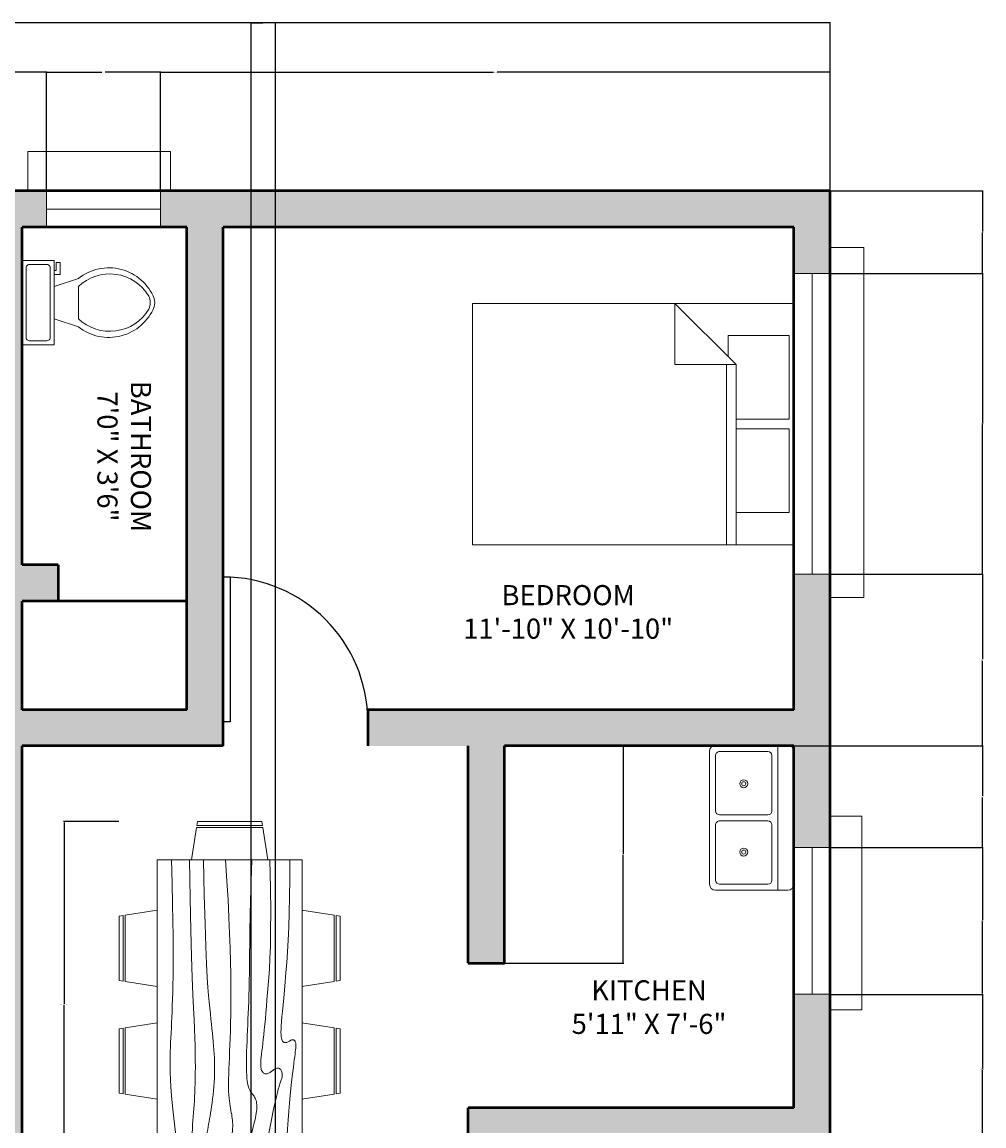
# Model space of a CAD drawing. Units: inches. Extents: x 2710 to 3197, y 524 to 1147.
# Tile 6 of 6: x 2957 to 3197, y 873 to 1147. Entities that reach past the tile are written whole.
import ezdxf

# ---------------------------------------------------------------- set-up
doc = ezdxf.new("R2010")
doc.units = ezdxf.units.IN
for name, color, linetype, lineweight in [('A-ANNO-DIMS', 2, 'Continuous', 18), ('A-AREA-IDEN', 7, 'Continuous', 25), ('A-DOOR', 3, 'Continuous', 25), ('A-FLOR-FIXT', 9, 'Continuous', 20), ('A-FURN', 8, 'Continuous', 18), ('A-GLAZ', 4, 'Continuous', 18), ('A-WALL', 7, 'Continuous', 50), ('A-WALL-PATT', 74, 'Continuous', 13)]:
    doc.layers.add(name, color=color, linetype=linetype, lineweight=lineweight)
doc.styles.get("Standard").update_dxf_attribs({"font": 'arial.ttf'})
doc.dimstyles.get("Standard").update_dxf_attribs({"dimtxt": 0.18, "dimasz": 0.18, "dimexe": 0.18, "dimexo": 0.0625, "dimgap": 0.09, "dimtad": 0, "dimtih": 1, "dimtoh": 1, "dimdec": 4, "dimzin": 0, "dimdsep": 46, "dimtxsty": 'Standard', "dimcen": 0.09, "dimadec": 0, "dimazin": 0, "dimtfac": 1, "dimtdec": 4, "dimtofl": 0, "dimtmove": 0, "dimatfit": 3, "dimfxl": 1, "dimtolj": 1, "dimtzin": 0, "dimarcsym": 0})

# ---------------------------------------------------------------- blocks, each defined once
blk = doc.blocks.new('*U4')
for p, q in [((0, 0), (0, -6)), ((36, 0), (36, -6))]:
    blk.add_line(p, q)
blk.add_lwpolyline([(0, 0), (0, 36), (1.75, 36), (1.75, 0)], close=True)
blk.add_arc((0, 0), 36, 0, 90)
blk = doc.blocks.new('Bed - Queen')
for p, q in [((0, -80.00003), (0, 0)), ((0, 0), (59.99999, 0)), ((59.99999, 0), (59.99999, -80.00003)), ((7.99999, -1.2), (28.79998, -1.2)), ((7.99999, -14.4), (7.99999, -1.2)), ((28.79998, -1.2), (28.79998, -14.4)), ((31.19999, -1.2), (51.99999, -1.2)), ((31.19999, -14.4), (31.19999, -1.2)), ((51.99999, -1.2), (51.99999, -16.4)), ((0, -14.4), (44.8, -14.4)), ((59.99999, -29.6), (44.8, -14.4)), ((44.8, -14.4), (44.8, -29.6)), ((51.99999, -16.4), (46.79936, -16.4)), ((44.8, -16.8), (0, -16.8)), ((44.8, -29.6), (59.99999, -29.6)), ((59.99999, -80.00003), (0, -80.00003))]:
    blk.add_line(p, q)
blk = doc.blocks.new('Toilet - top')
for p, q in [((9.5, -6), (9.5, -2)), ((-8, -8.5), (-8, -8)), ((-7, -8), (-7, -9.5)), ((-4, -8), (-6, -14)), ((4, -8), (6, -14)), ((-10, -8.5), (-8, -8.5)), ((-10, -9.5), (-10, -8.5)), ((-7, -9.5), (-10, -9.5)), ((4, -14), (-4, -14))]:
    blk.add_line(p, q)
blk.add_lwpolyline([(10.5, -8), (10.5, 0), (-10.5, 0), (-10.5, -8)], close=True)
for points in [[(-9.5, -2), (-9.5, -6)], [(8.5, -1), (-8.5, -1)], [(-8.5, -7), (8.5, -7)]]:
    blk.add_lwpolyline(points)
for centre, radius, start, end in [((-8.62, -1.88), 0.884, 81.8699, 188.1301), ((8.62, -1.88), 0.884, 351.8699, 98.1301), ((-8.62, -6.12), 0.884, 171.8699, 278.1301), ((8.62, -6.12), 0.884, 261.8699, 8.1301), ((3.52, -21.58), 12.17, 141.4691, 247.9714), ((4.2, -21.82), 11.33, 136.3677, 238.9468), ((-3.52, -21.58), 12.17, 292.0284, 38.5307), ((-4.2, -21.82), 11.33, 301.053, 43.6321), ((0, -27.88), 4, 245.7318, 294.2682), ((0, -29), 4, 254.8605, 285.1395)]:
    blk.add_arc(centre, radius, start, end)
blk = doc.blocks.new('Sink-double - 36 in top')
for p, q in [((-18, -4), (18, -4)), ((-0.75, -18.5), (-0.75, -6.5)), ((0.75, -6.5), (0.75, -18.5))]:
    blk.add_line(p, q)
for points in [[(-16.5, 0), (16.5, 0)], [(-18, -19.5), (-18, -1.5)], [(18, -1.5), (18, -19.5)], [(-16.5, -18.5), (-16.5, -6.5)], [(-15.5, -5.5), (-1.75, -5.5)], [(1.75, -5.5), (15.5, -5.5)], [(16.5, -6.5), (16.5, -18.5)], [(16.5, -21), (-16.5, -21)], [(-1.75, -19.5), (-15.5, -19.5)], [(15.5, -19.5), (1.75, -19.5)]]:
    blk.add_lwpolyline(points)
for centre, radius in [((-8.5, -12.5), 1), ((-8.5, -12.5), 0.5), ((8.5, -12.5), 1), ((8.5, -12.5), 0.5)]:
    blk.add_circle(centre, radius)
for centre, radius, start, end in [((-16.5, -1.5), 1.5, 90, 180), ((16.5, -1.5), 1.5, 0, 90), ((-15.5, -6.5), 1, 90, 180), ((-1.75, -6.5), 1, 0, 90), ((1.75, -6.5), 1, 90, 180), ((15.5, -6.5), 1, 0, 90), ((-15.5, -18.5), 1, 180, 270), ((-1.75, -18.5), 1, 270, 0), ((1.75, -18.5), 1, 180, 270), ((15.5, -18.5), 1, 270, 0), ((-16.5, -19.5), 1.5, 180, 270), ((16.5, -19.5), 1.5, 270, 0)]:
    blk.add_arc(centre, radius, start, end)
blk = doc.blocks.new('Dining Set - 36 x 72 in.')
for p, q in [((-22, 27.5), (-22.1562, 26.50042)), ((-22, 27.5), (-6, 27.5)), ((-5.8437, 26.49966), (-6, 27.5)), ((6, 27.5), (5.8438, 26.50042)), ((6, 27.5), (22, 27.5)), ((22.1563, 26.49966), (22, 27.5)), ((-22.2343, 26.00059), (-23.4847, 17.99762)), ((-22.2304, 26), (-5.7608, 26)), ((-5.8416, 26.5), (-22.1534, 26.5)), ((-4.5152, 17.99762), (-5.7655, 25.99926)), ((5.7657, 26.00059), (4.5153, 17.99762)), ((5.7696, 26), (22.2392, 26)), ((22.1584, 26.5), (5.8466, 26.5)), ((23.4848, 17.99762), (22.2345, 25.99926)), ((36, 18), (-36, 18)), ((-36, 18), (-36, -18)), ((36, -18), (36, 18)), ((-44.0006, 8.23428), (-35.9976, 9.48474)), ((44.0006, 8.23428), (35.9976, 9.48474)), ((-45.5, 8), (-44.5004, 8.15617)), ((-45.5, 8), (-45.5, -8)), ((-44.5, -8.15843), (-44.5, 8.15338)), ((-44, 8.23041), (-44, -8.23915)), ((44, 8.23041), (44, -8.23915)), ((44.5, -8.15843), (44.5, 8.15338)), ((45.5, 8), (44.5005, 8.15617)), ((45.5, 8), (45.5, -8)), ((-44.4997, -8.15631), (-45.5, -8)), ((-35.9976, -9.48476), (-43.9993, -8.2345)), ((35.9976, -9.48476), (43.9993, -8.2345)), ((44.4997, -8.15631), (45.5, -8)), ((-36, -18), (36, -18)), ((-22.2343, -26.0006), (-23.4847, -17.99762)), ((-4.5152, -17.99762), (-5.7655, -25.99928)), ((5.7657, -26.0006), (4.5153, -17.99762)), ((23.4848, -17.99762), (22.2345, -25.99928)), ((-22.2304, -26), (-5.7608, -26)), ((-22, -27.5), (-22.1562, -26.50044)), ((-5.8416, -26.5), (-22.1534, -26.5)), ((-5.8437, -26.49967), (-6, -27.5)), ((5.7696, -26), (22.2392, -26)), ((6, -27.5), (5.8438, -26.50044)), ((22.1584, -26.5), (5.8466, -26.5)), ((22.1563, -26.49967), (22, -27.5)), ((-22, -27.5), (-6, -27.5)), ((6, -27.5), (22, -27.5))]:
    blk.add_line(p, q)
for points in [[(-36, 15), (-31.1772, 14.97754), (-26.8079, 14.91406), (-22.8538, 14.81543), (-19.276, 14.6875), (-16.0362, 14.53613), (-13.0957, 14.36718), (-10.4159, 14.18652), (-7.9583, 14), (-5.6904, 13.81315), (-3.6035, 13.63021), (-1.6954, 13.45508), (0.0365, 13.29166), (1.5945, 13.14388), (2.9811, 13.01562), (4.1988, 12.9108), (5.25, 12.83333), (6.1393, 12.78613), (6.8802, 12.76823), (7.4883, 12.77767), (7.9792, 12.8125), (8.3685, 12.87077), (8.6719, 12.95052), (8.9049, 13.0498), (9.0833, 13.16666), (9.2205, 13.29899), (9.3216, 13.44401), (9.3895, 13.59879), (9.4271, 13.76041), (9.4373, 13.92594), (9.4232, 14.09245), (9.3875, 14.257), (9.3333, 14.41666), (9.2638, 14.56917), (9.1836, 14.71484), (9.0975, 14.85465), (9.0104, 14.98958), (8.9272, 15.1206), (8.8529, 15.2487), (8.7922, 15.37483), (8.75, 15.5), (8.7305, 15.62467), (8.7344, 15.74739), (8.7617, 15.86621), (8.8125, 15.97916), (8.8867, 16.08431), (8.9844, 16.17968), (9.1055, 16.26334), (9.25, 16.33333), (9.4189, 16.38802), (9.6172, 16.42708), (9.8506, 16.45052), (10.125, 16.45833), (10.4463, 16.45052), (10.8203, 16.42708), (11.2529, 16.38802), (11.75, 16.33333), (12.3184, 16.26318), (12.9694, 16.17838), (13.7151, 16.07991), (14.5677, 15.96875), (15.5395, 15.84586), (16.6426, 15.71224), (17.8893, 15.56884), (19.2917, 15.41666), (20.859, 15.25667), (22.5879, 15.08984), (24.4721, 14.91715), (26.5052, 14.73958), (28.6809, 14.5581), (30.9929, 14.3737), (33.4347, 14.18733), (36, 14)], [(-36, 10), (-28.9766, 10.14274), (-23.1725, 10.20442), (-18.4241, 10.19775), (-14.5677, 10.13541), (-11.4399, 10.03011), (-8.877, 9.89453), (-6.7154, 9.74137), (-4.7917, 9.58333), (-2.9698, 9.43082), (-1.2246, 9.28515), (0.4415, 9.14534), (2.026, 9.01041), (3.5266, 8.87939), (4.9408, 8.7513), (6.266, 8.62516), (7.5, 8.5), (8.6411, 8.37549), (9.6914, 8.2539), (10.6538, 8.13818), (11.5312, 8.03125), (12.3267, 7.93603), (13.043, 7.85547), (13.6831, 7.79248), (14.25, 7.75), (14.7471, 7.7303), (15.1797, 7.73307), (15.5537, 7.75732), (15.875, 7.80208), (16.1494, 7.86637), (16.3828, 7.94922), (16.5811, 8.04964), (16.75, 8.16666), (16.8944, 8.29915), (17.0143, 8.44531), (17.1089, 8.60319), (17.1771, 8.77083), (17.218, 8.94629), (17.2305, 9.1276), (17.2137, 9.31282), (17.1667, 9.5), (17.0895, 9.6875), (16.987, 9.875), (16.8649, 10.0625), (16.7292, 10.25), (16.5856, 10.4375), (16.4401, 10.625), (16.2985, 10.8125), (16.1667, 11), (16.05, 11.18733), (15.9518, 11.3737), (15.8752, 11.5581), (15.8229, 11.73958), (15.798, 11.91715), (15.8034, 12.08984), (15.842, 12.25667), (15.9167, 12.41666), (16.0295, 12.56836), (16.1784, 12.70833), (16.3605, 12.83268), (16.5729, 12.9375), (16.8127, 13.01888), (17.0768, 13.07291), (17.3625, 13.0957), (17.6667, 13.08333), (17.9894, 13.03312), (18.3418, 12.94726), (18.7382, 12.82918), (19.1927, 12.68229), (19.7195, 12.51001), (20.3327, 12.31575), (21.0465, 12.10294), (21.875, 11.875), (22.8357, 11.63354), (23.959, 11.37304), (25.2786, 11.08618), (26.8282, 10.76562), (28.6414, 10.40405), (30.752, 9.99414), (33.1936, 9.52856), (36, 9)], [(-36, 5.5), (-30.7157, 5.3348), (-26.069, 5.20963), (-21.9946, 5.11767), (-18.4271, 5.05208), (-15.3009, 5.00602), (-12.5508, 4.97265), (-10.1112, 4.94515), (-7.9167, 4.91666), (-5.909, 4.88167), (-4.0586, 4.83984), (-2.3429, 4.79215), (-0.7396, 4.73958), (0.7739, 4.6831), (2.22, 4.6237), (3.6213, 4.56233), (5, 4.5), (6.373, 4.43782), (7.7344, 4.3776), (9.0723, 4.32129), (10.375, 4.27083), (11.6309, 4.22819), (12.8281, 4.19531), (13.9551, 4.17415), (15, 4.16666), (15.954, 4.17448), (16.819, 4.19791), (17.6001, 4.23698), (18.3021, 4.29166), (18.9299, 4.36198), (19.4883, 4.44791), (19.9823, 4.54948), (20.4167, 4.66666), (20.7969, 4.79899), (21.1302, 4.94401), (21.4245, 5.09879), (21.6875, 5.26041), (21.9271, 5.42594), (22.1511, 5.59245), (22.3672, 5.757), (22.5834, 5.91666), (22.8065, 6.06868), (23.0404, 6.21093), (23.2879, 6.34147), (23.5521, 6.45833), (23.8358, 6.55957), (24.142, 6.64323), (24.4735, 6.70735), (24.8334, 6.75), (25.2235, 6.76969), (25.642, 6.76692), (26.0858, 6.74267), (26.5521, 6.69791), (27.0379, 6.63362), (27.5404, 6.55078), (28.0565, 6.45036), (28.5834, 6.33333), (29.1242, 6.19987), (29.7071, 6.04687), (30.3661, 5.87044), (31.1354, 5.66666), (32.0493, 5.43164), (33.142, 5.16146), (34.4475, 4.85221), (36, 4.5)], [(-36, -1), (-30.7915, -0.6591), (-26.0195, -0.38216), (-21.6519, -0.16284), (-17.6563, 0.00521), (-14.0005, 0.12833), (-10.6523, 0.21289), (-7.5796, 0.26522), (-4.75, 0.29166), (-2.134, 0.29793), (0.2878, 0.28711), (2.5317, 0.26163), (4.6146, 0.22396), (6.5529, 0.17651), (8.3633, 0.12174), (10.0623, 0.06209), (11.6667, 0), (13.1899, -0.06201), (14.6341, -0.1211), (15.9982, -0.17432), (17.2813, -0.21875), (18.4823, -0.25147), (19.6003, -0.26953), (20.6343, -0.27002), (21.5834, -0.25), (22.4481, -0.20768), (23.2357, -0.14584), (23.9549, -0.06836), (24.6146, 0.02083), (25.2235, 0.11784), (25.7904, 0.21875), (26.3241, 0.31966), (26.8334, 0.41666), (27.3265, 0.50618), (27.8099, 0.58593), (28.2894, 0.65397), (28.7709, 0.70833), (29.2601, 0.74707), (29.763, 0.76823), (30.2855, 0.76985), (30.8334, 0.75), (31.4088, 0.70784), (31.9994, 0.64713), (32.589, 0.57275), (33.1615, 0.48958), (33.7008, 0.4025), (34.1908, 0.3164), (34.6153, 0.23616), (34.9584, 0.16666), (35.2099, 0.11165), (35.3848, 0.07031), (35.504, 0.04069), (35.5886, 0.02083), (35.6594, 0.00879), (35.7377, 0.0026), (35.8442, 0.00032), (36, 0)], [(-36, -6.5), (-27.1843, -6.31267), (-20.084, -6.1263), (-14.469, -5.9419), (-10.1094, -5.76042), (-6.7752, -5.58285), (-4.2363, -5.41016), (-2.2629, -5.24333), (-0.625, -5.08334), (0.8708, -4.93099), (2.2715, -4.78646), (3.5872, -4.64974), (4.8281, -4.52084), (6.0046, -4.39974), (7.127, -4.28646), (8.2053, -4.18099), (9.25, -4.08334), (10.2705, -3.99382), (11.2734, -3.91407), (12.2647, -3.84603), (13.25, -3.79167), (14.2354, -3.75293), (15.2266, -3.73177), (16.2295, -3.73015), (17.25, -3.75), (18.2912, -3.79248), (19.3451, -3.85547), (20.4009, -3.93604), (21.4479, -4.03125), (22.4754, -4.13819), (23.4727, -4.25391), (24.4289, -4.37549), (25.3334, -4.5), (26.1785, -4.62492), (26.9694, -4.74935), (27.7145, -4.87281), (28.4219, -4.99479), (29.1, -5.11483), (29.7572, -5.23242), (30.4016, -5.34709), (31.0417, -5.45834), (31.6837, -5.56437), (32.3262, -5.65821), (32.9658, -5.73153), (33.599, -5.77604), (34.2224, -5.78345), (34.8327, -5.74545), (35.4264, -5.65373), (36, -5.5)], [(-36, -10), (-26.4022, -9.81299), (-18.4675, -9.62891), (-11.9839, -9.45069), (-6.7396, -9.28125), (-2.5226, -9.12354), (0.8789, -8.98047), (3.6769, -8.85498), (6.0833, -8.75), (8.2767, -8.66765), (10.3021, -8.60677), (12.1712, -8.56543), (13.8958, -8.54167), (15.4876, -8.53353), (16.9583, -8.53907), (18.3197, -8.55632), (19.5834, -8.58334), (20.7616, -8.61841), (21.8685, -8.66081), (22.9188, -8.71004), (23.9271, -8.76563), (24.9081, -8.82707), (25.8763, -8.89388), (26.8465, -8.96558), (27.8334, -9.04167), (28.8474, -9.12118), (29.8828, -9.20117), (30.93, -9.27824), (31.9792, -9.34896), (33.0205, -9.40991), (34.0443, -9.45768), (35.0407, -9.48885), (36, -9.5)], [(-36, -14.5), (-30.0881, -14.33513), (-25.0332, -14.21224), (-20.7312, -14.12647), (-17.0781, -14.07292), (-13.97, -14.04671), (-11.3027, -14.04297), (-8.9724, -14.05681), (-6.875, -14.08334), (-4.9224, -14.11833), (-3.0905, -14.16016), (-1.3709, -14.20785), (0.2448, -14.26042), (1.7647, -14.3169), (3.1973, -14.3763), (4.5507, -14.43767), (5.8333, -14.5), (7.0554, -14.5621), (8.235, -14.62175), (9.3922, -14.67652), (10.5469, -14.72396), (11.7192, -14.76164), (12.929, -14.78711), (14.1965, -14.79794), (15.5417, -14.79167), (16.9933, -14.76424), (18.6152, -14.70508), (20.4804, -14.60197), (22.6615, -14.44271), (25.2312, -14.21509), (28.2624, -13.9069), (31.8277, -13.50594), (36, -13)]]:
    blk.add_lwpolyline(points)
blk = doc.blocks.new('*D26')
at = {"layer": 'A-ANNO-DIMS', "color": 0, "lineweight": -2, "transparency": 16777216}
for p, q in [((2981.42, 948.17), (2967.65, 948.17)), ((2967.83, 947.99), (2967.83, 902.86)), ((2967.83, 857.35), (2967.83, 902.49)), ((2981.42, 857.17), (2967.65, 857.17))]:
    blk.add_line(p, q, dxfattribs=at)
at = {"layer": 'A-ANNO-DIMS', "color": 0, "transparency": 16777216}
for points in [[(2967.8, 947.99), (2967.86, 947.99), (2967.83, 948.17)], [(2967.8, 857.35), (2967.86, 857.35), (2967.83, 857.17)]]:
    blk.add_solid(points, dxfattribs=at)
at = {"layer": 'Defpoints', "color": 0, "transparency": 16777216}
for p in [(2981.48, 948.17), (2967.83, 857.17), (2981.48, 857.17)]:
    blk.add_point(p, dxfattribs=at)
at = {"layer": 'A-ANNO-DIMS', "color": 0, "transparency": 16777216, "insert": (2967.83, 902.67), "char_height": 0.18, "attachment_point": 5}
blk.add_mtext('\\A1;DINING SET 91 TYP.', dxfattribs=at)
blk = doc.blocks.new('*D34')
at = {"layer": 'A-ANNO-DIMS', "color": 0, "lineweight": -2, "transparency": 16777216}
for p, q in [((2747.35, 1105.06), (2747.35, 1146.99)), ((2747.53, 1146.81), (2952.57, 1146.81)), ((3158.17, 1146.81), (2953.12, 1146.81)), ((3158.35, 1105.06), (3158.35, 1146.99))]:
    blk.add_line(p, q, dxfattribs=at)
at = {"layer": 'A-ANNO-DIMS', "color": 0, "transparency": 16777216}
for points in [[(2747.53, 1146.84), (2747.53, 1146.78), (2747.35, 1146.81)], [(3158.17, 1146.84), (3158.17, 1146.78), (3158.35, 1146.81)]]:
    blk.add_solid(points, dxfattribs=at)
at = {"layer": 'Defpoints', "color": 0, "transparency": 16777216}
for p in [(3158.35, 1146.81), (2747.35, 1105), (3158.35, 1105)]:
    blk.add_point(p, dxfattribs=at)
at = {"layer": 'A-ANNO-DIMS', "color": 0, "transparency": 16777216, "insert": (2952.85, 1146.81), "char_height": 0.18, "attachment_point": 5}
blk.add_mtext('\\A1;411', dxfattribs=at)
blk = doc.blocks.new('*D40')
at = {"layer": 'A-ANNO-DIMS', "color": 0, "lineweight": -2, "transparency": 16777216}
for p, q in [((2940.7, 1105.06), (2940.7, 1134.68)), ((2940.88, 1134.5), (2951.61, 1134.5)), ((2963.27, 1134.5), (2952.54, 1134.5)), ((2963.45, 1105.06), (2963.45, 1134.68))]:
    blk.add_line(p, q, dxfattribs=at)
at = {"layer": 'A-ANNO-DIMS', "color": 0, "transparency": 16777216}
for points in [[(2940.88, 1134.53), (2940.88, 1134.47), (2940.7, 1134.5)], [(2963.27, 1134.53), (2963.27, 1134.47), (2963.45, 1134.5)]]:
    blk.add_solid(points, dxfattribs=at)
at = {"layer": 'Defpoints', "color": 0, "transparency": 16777216}
for p in [(2963.45, 1134.5), (2940.7, 1105), (2963.45, 1105)]:
    blk.add_point(p, dxfattribs=at)
at = {"layer": 'A-ANNO-DIMS', "color": 0, "transparency": 16777216, "insert": (2952.08, 1134.5), "char_height": 0.18, "attachment_point": 5}
blk.add_mtext('\\A1;22.746', dxfattribs=at)
blk = doc.blocks.new('*D41')
at = {"layer": 'A-ANNO-DIMS', "color": 0, "lineweight": -2, "transparency": 16777216}
for p, q in [((2963.45, 1105.06), (2963.45, 1134.68)), ((2963.63, 1134.5), (2977.22, 1134.5)), ((2991.6, 1134.5), (2978.01, 1134.5)), ((2991.78, 1105.06), (2991.78, 1134.68))]:
    blk.add_line(p, q, dxfattribs=at)
at = {"layer": 'A-ANNO-DIMS', "color": 0, "transparency": 16777216}
for points in [[(2963.63, 1134.53), (2963.63, 1134.47), (2963.45, 1134.5)], [(2991.6, 1134.53), (2991.6, 1134.47), (2991.78, 1134.5)]]:
    blk.add_solid(points, dxfattribs=at)
at = {"layer": 'Defpoints', "color": 0, "transparency": 16777216}
for p in [(2991.78, 1134.5), (2963.45, 1105), (2991.78, 1105)]:
    blk.add_point(p, dxfattribs=at)
at = {"layer": 'A-ANNO-DIMS', "color": 0, "transparency": 16777216, "insert": (2977.61, 1134.5), "char_height": 0.18, "attachment_point": 5}
blk.add_mtext('\\A1;28.33', dxfattribs=at)
blk = doc.blocks.new('*D42')
at = {"layer": 'A-ANNO-DIMS', "color": 0, "lineweight": -2, "transparency": 16777216}
for p, q in [((2991.78, 1105.06), (2991.78, 1134.68)), ((2991.96, 1134.5), (3074.61, 1134.5)), ((3158.17, 1134.5), (3075.52, 1134.5)), ((3158.35, 1105.06), (3158.35, 1134.68))]:
    blk.add_line(p, q, dxfattribs=at)
at = {"layer": 'A-ANNO-DIMS', "color": 0, "transparency": 16777216}
for points in [[(2991.96, 1134.53), (2991.96, 1134.47), (2991.78, 1134.5)], [(3158.17, 1134.53), (3158.17, 1134.47), (3158.35, 1134.5)]]:
    blk.add_solid(points, dxfattribs=at)
at = {"layer": 'Defpoints', "color": 0, "transparency": 16777216}
for p in [(3158.35, 1134.5), (2991.78, 1105), (3158.35, 1105)]:
    blk.add_point(p, dxfattribs=at)
at = {"layer": 'A-ANNO-DIMS', "color": 0, "transparency": 16777216, "insert": (3075.06, 1134.5), "char_height": 0.18, "attachment_point": 5}
blk.add_mtext('\\A1;166.57', dxfattribs=at)
blk = doc.blocks.new('*D64')
at = {"layer": 'A-ANNO-DIMS', "color": 0, "lineweight": -2, "transparency": 16777216}
for p, q in [((3158.41, 905.22), (3196.41, 905.22)), ((3196.23, 905.04), (3196.23, 886.79)), ((3196.23, 868.18), (3196.23, 886.43)), ((3149.41, 868), (3196.41, 868))]:
    blk.add_line(p, q, dxfattribs=at)
at = {"layer": 'A-ANNO-DIMS', "color": 0, "transparency": 16777216}
for points in [[(3196.2, 905.04), (3196.26, 905.04), (3196.23, 905.22)], [(3196.2, 868.18), (3196.26, 868.18), (3196.23, 868)]]:
    blk.add_solid(points, dxfattribs=at)
at = {"layer": 'Defpoints', "color": 0, "transparency": 16777216}
for p in [(3158.35, 905.22), (3196.23, 905.22), (3149.35, 868)]:
    blk.add_point(p, dxfattribs=at)
at = {"layer": 'A-ANNO-DIMS', "color": 0, "transparency": 16777216, "insert": (3196.23, 886.61), "char_height": 0.18, "attachment_point": 5}
blk.add_mtext('\\A1;37.22', dxfattribs=at)
blk = doc.blocks.new('*D65')
at = {"layer": 'A-ANNO-DIMS', "color": 0, "lineweight": -2, "transparency": 16777216}
for p, q in [((3158.41, 941.76), (3196.41, 941.76)), ((3196.23, 941.58), (3196.23, 923.67)), ((3196.23, 905.4), (3196.23, 923.31)), ((3158.41, 905.22), (3196.41, 905.22))]:
    blk.add_line(p, q, dxfattribs=at)
at = {"layer": 'A-ANNO-DIMS', "color": 0, "transparency": 16777216}
for points in [[(3196.2, 941.58), (3196.26, 941.58), (3196.23, 941.76)], [(3196.2, 905.4), (3196.26, 905.4), (3196.23, 905.22)]]:
    blk.add_solid(points, dxfattribs=at)
at = {"layer": 'Defpoints', "color": 0, "transparency": 16777216}
for p in [(3158.35, 941.76), (3196.23, 941.76), (3158.35, 905.22)]:
    blk.add_point(p, dxfattribs=at)
at = {"layer": 'A-ANNO-DIMS', "color": 0, "transparency": 16777216, "insert": (3196.23, 923.49), "char_height": 0.18, "attachment_point": 5}
blk.add_mtext('\\A1;36.53', dxfattribs=at)
blk = doc.blocks.new('*D66')
at = {"layer": 'A-ANNO-DIMS', "color": 0, "lineweight": -2, "transparency": 16777216}
for p, q in [((3149.41, 967), (3196.41, 967)), ((3196.23, 966.82), (3196.23, 954.56)), ((3196.23, 941.94), (3196.23, 954.2)), ((3158.41, 941.76), (3196.41, 941.76))]:
    blk.add_line(p, q, dxfattribs=at)
at = {"layer": 'A-ANNO-DIMS', "color": 0, "transparency": 16777216}
for points in [[(3196.2, 966.82), (3196.26, 966.82), (3196.23, 967)], [(3196.2, 941.94), (3196.26, 941.94), (3196.23, 941.76)]]:
    blk.add_solid(points, dxfattribs=at)
at = {"layer": 'Defpoints', "color": 0, "transparency": 16777216}
for p in [(3149.35, 967), (3196.23, 967), (3158.35, 941.76)]:
    blk.add_point(p, dxfattribs=at)
at = {"layer": 'A-ANNO-DIMS', "color": 0, "transparency": 16777216, "insert": (3196.23, 954.38), "char_height": 0.18, "attachment_point": 5}
blk.add_mtext('\\A1;25.245', dxfattribs=at)
blk = doc.blocks.new('*D67')
at = {"layer": 'A-ANNO-DIMS', "color": 0, "lineweight": -2, "transparency": 16777216}
for p, q in [((3158.41, 1009.7), (3196.41, 1009.7)), ((3196.23, 1009.52), (3196.23, 988.53)), ((3196.23, 967.18), (3196.23, 988.17)), ((3149.41, 967), (3196.41, 967))]:
    blk.add_line(p, q, dxfattribs=at)
at = {"layer": 'A-ANNO-DIMS', "color": 0, "transparency": 16777216}
for points in [[(3196.2, 1009.52), (3196.26, 1009.52), (3196.23, 1009.7)], [(3196.2, 967.18), (3196.26, 967.18), (3196.23, 967)]]:
    blk.add_solid(points, dxfattribs=at)
at = {"layer": 'Defpoints', "color": 0, "transparency": 16777216}
for p in [(3158.35, 1009.7), (3196.23, 1009.7), (3149.35, 967)]:
    blk.add_point(p, dxfattribs=at)
at = {"layer": 'A-ANNO-DIMS', "color": 0, "transparency": 16777216, "insert": (3196.23, 988.35), "char_height": 0.18, "attachment_point": 5}
blk.add_mtext('\\A1;42.7', dxfattribs=at)
blk = doc.blocks.new('*D68')
at = {"layer": 'A-ANNO-DIMS', "color": 0, "lineweight": -2, "transparency": 16777216}
for p, q in [((3158.41, 1084.46), (3196.41, 1084.46)), ((3196.23, 1084.28), (3196.23, 1047.26)), ((3196.23, 1009.88), (3196.23, 1046.9)), ((3158.41, 1009.7), (3196.41, 1009.7))]:
    blk.add_line(p, q, dxfattribs=at)
at = {"layer": 'A-ANNO-DIMS', "color": 0, "transparency": 16777216}
for points in [[(3196.2, 1084.28), (3196.26, 1084.28), (3196.23, 1084.46)], [(3196.2, 1009.88), (3196.26, 1009.88), (3196.23, 1009.7)]]:
    blk.add_solid(points, dxfattribs=at)
at = {"layer": 'Defpoints', "color": 0, "transparency": 16777216}
for p in [(3158.35, 1084.46), (3196.23, 1084.46), (3158.35, 1009.7)]:
    blk.add_point(p, dxfattribs=at)
at = {"layer": 'A-ANNO-DIMS', "color": 0, "transparency": 16777216, "insert": (3196.23, 1047.08), "char_height": 0.18, "attachment_point": 5}
blk.add_mtext('\\A1;74.76', dxfattribs=at)
blk = doc.blocks.new('*D69')
at = {"layer": 'A-ANNO-DIMS', "color": 0, "lineweight": -2, "transparency": 16777216}
for p, q in [((3158.41, 1105), (3196.41, 1105)), ((3196.23, 1104.82), (3196.23, 1094.91)), ((3196.23, 1084.64), (3196.23, 1094.55)), ((3158.41, 1084.46), (3196.41, 1084.46))]:
    blk.add_line(p, q, dxfattribs=at)
at = {"layer": 'A-ANNO-DIMS', "color": 0, "transparency": 16777216}
for points in [[(3196.2, 1104.82), (3196.26, 1104.82), (3196.23, 1105)], [(3196.2, 1084.64), (3196.26, 1084.64), (3196.23, 1084.46)]]:
    blk.add_solid(points, dxfattribs=at)
at = {"layer": 'Defpoints', "color": 0, "transparency": 16777216}
for p in [(3158.35, 1105), (3196.23, 1105), (3158.35, 1084.46)]:
    blk.add_point(p, dxfattribs=at)
at = {"layer": 'A-ANNO-DIMS', "color": 0, "transparency": 16777216, "insert": (3196.23, 1094.73), "char_height": 0.18, "attachment_point": 5}
blk.add_mtext('\\A1;20.54', dxfattribs=at)
blk = doc.blocks.new('*D79')
at = {"layer": 'A-ANNO-DIMS', "color": 0, "lineweight": -2, "transparency": 16777216}
for p, q in [((3014.35, 787.06), (3014.35, 1146.99)), ((3014.53, 1146.81), (3017.2, 1146.81)), ((3020.17, 1146.81), (3017.5, 1146.81)), ((3020.35, 796.06), (3020.35, 1146.99))]:
    blk.add_line(p, q, dxfattribs=at)
at = {"layer": 'A-ANNO-DIMS', "color": 0, "transparency": 16777216}
for points in [[(3014.53, 1146.84), (3014.53, 1146.78), (3014.35, 1146.81)], [(3020.17, 1146.84), (3020.17, 1146.78), (3020.35, 1146.81)]]:
    blk.add_solid(points, dxfattribs=at)
at = {"layer": 'Defpoints', "color": 0, "transparency": 16777216}
for p in [(3020.35, 1146.81), (3020.35, 796), (3014.35, 787)]:
    blk.add_point(p, dxfattribs=at)
at = {"layer": 'A-ANNO-DIMS', "color": 0, "transparency": 16777216, "insert": (3017.35, 1146.81), "char_height": 0.18, "attachment_point": 5}
blk.add_mtext('\\A1;6', dxfattribs=at)
blk = doc.blocks.new('*D84')
at = {"layer": 'A-ANNO-DIMS', "color": 0, "lineweight": -2, "transparency": 16777216}
for p, q in [((3077.41, 967), (3107.03, 967)), ((3106.85, 966.82), (3106.85, 940.18)), ((3106.85, 913.18), (3106.85, 939.82)), ((3077.41, 913), (3107.03, 913))]:
    blk.add_line(p, q, dxfattribs=at)
at = {"layer": 'A-ANNO-DIMS', "color": 0, "transparency": 16777216}
for points in [[(3106.82, 966.82), (3106.88, 966.82), (3106.85, 967)], [(3106.82, 913.18), (3106.88, 913.18), (3106.85, 913)]]:
    blk.add_solid(points, dxfattribs=at)
at = {"layer": 'Defpoints', "color": 0, "transparency": 16777216}
for p in [(3077.35, 967), (3077.35, 913), (3106.85, 913)]:
    blk.add_point(p, dxfattribs=at)
at = {"layer": 'A-ANNO-DIMS', "color": 0, "transparency": 16777216, "insert": (3106.85, 940), "char_height": 0.18, "attachment_point": 5}
blk.add_mtext('\\A1;54', dxfattribs=at)

msp = doc.modelspace()

# ---------------------------------------------------------------- hatches: boundary and pattern name
at = {"layer": 'A-WALL-PATT'}
h = msp.add_hatch(color=256, dxfattribs=at)
h.dxf.hatch_style = 1
h.paths.add_polyline_path([(2898.3484, 1096.0017), (2898.3484, 967.0017), (2948.3484, 967.0017), (2948.3484, 787.0017), (2957.3484, 787.0017), (2957.3484, 793.0017), (2957.3484, 833.0017), (2957.3484, 967.0017), (3007.3484, 967.0017), (3007.3484, 973.0017), (3007.3484, 1009.0017), (3007.3484, 1096.0017), (3149.3484, 1096.0017), (3149.3484, 1084.4601), (3158.3484, 1084.4601), (3158.3484, 1105.0017), (2991.781, 1105.0017), (2991.781, 1096.0017), (2998.3484, 1096.0017), (2998.3484, 976.0017), (2957.3484, 976.0017), (2957.3484, 1003.0017), (2966.3484, 1003.0017), (2966.3484, 1012.0017), (2957.3484, 1012.0017), (2957.3484, 1096.0017), (2963.4487, 1096.0017), (2963.4487, 1105.0017), (2940.703, 1105.0017), (2940.703, 1096.0017), (2948.3484, 1096.0017), (2948.3484, 1012.0017), (2939.3484, 1012.0017), (2939.3484, 1003.0017), (2948.3484, 1003.0017), (2948.3484, 976.0017), (2907.3484, 976.0017), (2907.3484, 1096.0017), (2916.9598, 1096.0017), (2916.9598, 1105.0017), (2857.03, 1105.0017), (2857.03, 1096.0017)])
h.paths.add_polyline_path([(2789.8274, 1096.0017), (2789.8274, 1105.0017), (2747.3484, 1105.0017), (2747.3484, 943.327), (2756.3484, 943.327), (2756.3484, 967.0017), (2828.3484, 967.0017), (2828.3484, 909.0017), (2837.3484, 909.0017), (2837.3484, 967.0017), (2862.3484, 967.0017), (2862.3484, 973.0017), (2862.3484, 976.0017), (2756.3484, 976.0017), (2756.3484, 1096.0017)])
h.paths.add_polyline_path([(2828.3484, 868.0017), (2828.3484, 830.0017), (2837.3484, 830.0017), (2837.3484, 877.0017), (2756.3484, 877.0017), (2756.3484, 904.8338), (2747.3484, 904.8338), (2747.3484, 858.8554), (2756.3484, 858.8554), (2756.3484, 868.0017)])
h.paths.add_polyline_path([(2747.3484, 742.5572), (2756.3484, 742.5572), (2756.3484, 787.0017), (2849.3484, 787.0017), (2849.3484, 796.0017), (2837.3484, 796.0017), (2837.3484, 802.0017), (2831.3484, 802.0017), (2828.3484, 802.0017), (2828.3484, 796.0017), (2756.3484, 796.0017), (2756.3484, 819.3052), (2747.3484, 819.3052)])
h.paths.add_polyline_path([(2756.3484, 643.0017), (2756.3484, 672.4477), (2747.3484, 672.4477), (2747.3484, 565.0017), (2825.5051, 565.0017), (2825.5051, 574.0017), (2756.3484, 574.0017), (2756.3484, 634.0017), (2891.3484, 634.0017), (2891.3484, 787.0017), (2908.3484, 787.0017), (2908.3484, 793.0017), (2908.3484, 796.0017), (2891.3484, 796.0017), (2885.3484, 796.0017), (2885.3484, 790.0017), (2885.3484, 754.0017), (2885.3484, 643.0017)])
h.paths.add_polyline_path([(2924.8484, 565.0017), (2924.8484, 571.0017), (2924.8484, 574.0017), (2872.3715, 574.0017), (2872.3715, 565.0017)])
h.paths.add_polyline_path([(2984.8484, 574.0017), (2984.8484, 571.0017), (2984.8484, 565.0017), (3050.793, 565.0017), (3050.793, 574.0017)])
h.paths.add_polyline_path([(3158.3484, 565.0017), (3158.3484, 685.5326), (3149.3484, 685.5326), (3149.3484, 675.4542), (3149.3484, 643.0017), (3020.3484, 643.0017), (3020.3484, 796.0017), (3014.3484, 796.0017), (2997.3484, 796.0017), (2997.3484, 787.0017), (3014.3484, 787.0017), (3014.3484, 634.0017), (3149.3484, 634.0017), (3149.3484, 574.0017), (3104.3903, 574.0017), (3104.3903, 565.0017)])
h.paths.add_polyline_path([(3149.3484, 787.0017), (3149.3484, 746.9465), (3158.3484, 746.9465), (3158.3484, 820.3805), (3149.3484, 820.3805), (3149.3484, 796.0017), (3077.3484, 796.0017), (3077.3484, 802.0017), (3074.3484, 802.0017), (3068.3484, 802.0017), (3068.3484, 796.0017), (3056.3484, 796.0017), (3056.3484, 790.0017), (3056.3484, 787.0017)])
h.paths.add_polyline_path([(3158.3484, 905.224), (3149.3484, 905.224), (3149.3484, 877.0017), (3068.3484, 877.0017), (3068.3484, 838.0017), (3074.3484, 838.0017), (3077.3484, 838.0017), (3077.3484, 868.0017), (3149.3484, 868.0017), (3149.3484, 852.3022), (3158.3484, 852.3022)], flags=17)
h.paths.add_polyline_path([(3099.2867, 814.3126), (3142.0289, 814.3126), (3142.0289, 832.97), (3099.2867, 832.97)], flags=25)
h.paths.add_polyline_path([(2981.8144, 832.8032), (3033.605, 832.8032), (3033.605, 851.4605), (2981.8144, 851.4605)], flags=25)
h = msp.add_hatch(color=256, dxfattribs=at)
h.dxf.hatch_style = 1
h.paths.add_polyline_path([(3158.3484, 1009.704), (3149.3484, 1009.704), (3149.3484, 976.0017), (3043.3484, 976.0017), (3043.3484, 967.0017), (3068.3484, 967.0017), (3068.3484, 913.0017), (3077.3484, 913.0017), (3077.3484, 967.0017), (3149.3484, 967.0017), (3149.3484, 941.7567), (3158.3484, 941.7567)])

# ---------------------------------------------------------------- linework, layer by layer
at = {"layer": 'A-GLAZ'}
for p, q in [((2958.7826, 1105.0017), (2958.7826, 1114.8131)), ((2958.7826, 1114.8131), (2994.2934, 1114.8131)), ((2994.2934, 1114.8131), (2994.2934, 1105.0017)), ((2963.4487, 1096.0017), (2963.4487, 1105.0017)), ((2991.781, 1096.0017), (2991.781, 1105.0017)), ((2991.781, 1100.5017), (2963.4487, 1100.5017)), ((3158.3484, 1090.968), (3166.7275, 1090.968)), ((3166.7275, 1090.968), (3166.7275, 1003.9147)), ((3149.3484, 1084.4601), (3158.3484, 1084.4601)), ((3153.8484, 1009.704), (3153.8484, 1084.4601)), ((3149.3484, 1009.704), (3158.3484, 1009.704)), ((3166.7275, 1003.9147), (3158.3484, 1003.9147)), ((3158.3484, 949.4986), (3166.2314, 949.4986)), ((3166.2314, 949.4986), (3166.2314, 901.407)), ((3149.3484, 941.7567), (3158.3484, 941.7567)), ((3153.8484, 905.224), (3153.8484, 941.7567)), ((3149.3484, 905.224), (3158.3484, 905.224)), ((3166.2314, 901.407), (3158.3484, 901.407))]:
    msp.add_line(p, q, dxfattribs=at)
at = {"layer": 'A-WALL'}
for p, q in [((3158.3484, 1105.0017), (2747.3484, 1105.0017)), ((3158.3484, 565.0017), (3158.3484, 1105.0017)), ((2998.3484, 1096.0017), (2957.3484, 1096.0017)), ((2957.3484, 1012.0017), (2957.3484, 1096.0017)), ((2998.3484, 976.0017), (2998.3484, 1096.0017)), ((3149.3484, 1096.0017), (3007.3484, 1096.0017)), ((3007.3484, 967.0017), (3007.3484, 1096.0017)), ((3149.3484, 976.0017), (3149.3484, 1096.0017)), ((2966.3484, 1012.0017), (2957.3484, 1012.0017)), ((2966.3484, 1012.0017), (2966.3484, 1003.0017)), ((2998.3484, 1003.0017), (2957.3484, 1003.0017)), ((2957.3484, 976.0017), (2957.3484, 1003.0017)), ((2998.3484, 976.0017), (2957.3484, 976.0017)), ((3149.3484, 976.0017), (3043.3484, 976.0017)), ((3043.3484, 976.0017), (3043.3484, 967.0017)), ((2957.3484, 787.0017), (2957.3484, 967.0017)), ((3007.3484, 967.0017), (2957.3484, 967.0017)), ((3068.3484, 913.0017), (3068.3484, 967.0017)), ((3149.3484, 967.0017), (3077.3484, 967.0017)), ((3077.3484, 913.0017), (3077.3484, 967.0017)), ((3149.3484, 877.0017), (3149.3484, 967.0017)), ((3068.3484, 913.0017), (3077.3484, 913.0017)), ((3149.3484, 877.0017), (3068.3484, 877.0017)), ((3068.3484, 838.0017), (3068.3484, 877.0017))]:
    msp.add_line(p, q, dxfattribs=at)

# ---------------------------------------------------------------- block references
at = {"layer": 'A-DOOR'}
msp.add_blockref('*U4', (3007.3484, 973.0017), dxfattribs=at)
at = {"layer": 'A-FLOR-FIXT', "xscale": -1}
for name, p, rotation in [('Toilet - top', (2957.3484, 1077.2281), 90), ('Sink-double - 36 in top', (3149.3484, 949.0976), 270)]:
    msp.add_blockref(name, p, dxfattribs=dict(at, rotation=rotation))
at = {"layer": 'A-FURN', "xscale": -1, "rotation": 270}
msp.add_blockref('Bed - Queen', (3149.3484, 1017.0333), dxfattribs=at)
at = {"layer": 'A-FURN', "rotation": 270}
msp.add_blockref('Dining Set - 36 x 72 in.', (3008.9802, 902.6723), dxfattribs=at)

# ---------------------------------------------------------------- texts
at = {"layer": 'A-AREA-IDEN', "insert": (2989.4254, 1067.79), "char_height": 5, "attachment_point": 1, "rotation": 270}
msp.add_mtext_dynamic_manual_height_columns('\\pxqc;BATHROOM\\P7\'0" X 3\'6"', width=57.655828, gutter_width=12.5, heights=[0], dxfattribs=at)
at = {"layer": 'A-AREA-IDEN', "char_height": 5, "attachment_point": 1}
for s, insert in [('\\pxqc;BEDROOM\\P11\'-10" X 10\'-10"', (3064.3608, 1006.989)), ('\\pxqc;KITCHEN\\P5\'11" X 7\'-6"', (3084.4706, 908.7096))]:
    msp.add_mtext_dynamic_manual_height_columns(s, width=57.655828, gutter_width=12.5, heights=[0], dxfattribs=dict(at, insert=insert))

# ---------------------------------------------------------------- dimensions: what is measured, and where the dimension line sits
at = {"layer": 'A-ANNO-DIMS'}
for base, p1, p2, override, picture, middle in [((3158.3484, 1146.8081), (2747.3484, 1105.0017), (3158.3484, 1105.0017), {"dimdec": 0, "dimlfac": 1, "dimrnd": 0, "dimzin": 0, "dimdsep": 46, "dimlunit": 2}, '*D34', (2952.8484, 1146.8081)), ((3020.3484, 1146.8081), (3014.3484, 787.0017), (3020.3484, 796.0017), {"dimdec": 0, "dimlfac": 1, "dimrnd": 0, "dimzin": 0, "dimdsep": 46, "dimlunit": 2}, '*D79', (3017.3484, 1146.8081)), ((2963.4487, 1134.5017), (2940.703, 1105.0017), (2963.4487, 1105.0017), {"dimdec": 3, "dimlfac": 1, "dimrnd": 0, "dimzin": 0, "dimdsep": 46, "dimlunit": 2}, '*D40', (2952.0759, 1134.5017)), ((2991.781, 1134.5017), (2963.4487, 1105.0017), (2991.781, 1105.0017), {"dimdec": 2, "dimlfac": 1, "dimrnd": 0, "dimzin": 0, "dimdsep": 46, "dimlunit": 2}, '*D41', (2977.6149, 1134.5017)), ((3158.3484, 1134.5017), (2991.781, 1105.0017), (3158.3484, 1105.0017), {"dimdec": 2, "dimlfac": 1, "dimrnd": 0, "dimzin": 0, "dimdsep": 46, "dimlunit": 2}, '*D42', (3075.0647, 1134.5017))]:
    dim = msp.add_linear_dim(base=base, p1=p1, p2=p2, dimstyle='Standard', override=override, dxfattribs=at)
    dim.commit()
    dim.dimension.update_dxf_attribs({"geometry": picture, "text_midpoint": middle})
for base, p1, p2, angle, override, picture, middle in [((3196.2275, 1105.0017), (3158.3484, 1084.4601), (3158.3484, 1105.0017), 90, {"dimdec": 2, "dimlfac": 1, "dimrnd": 0, "dimzin": 0, "dimdsep": 46, "dimlunit": 2}, '*D69', (3196.2275, 1094.7309)), ((3196.2275, 1084.4601), (3158.3484, 1009.704), (3158.3484, 1084.4601), 90, {"dimdec": 2, "dimlfac": 1, "dimrnd": 0, "dimzin": 0, "dimdsep": 46, "dimlunit": 2}, '*D68', (3196.2275, 1047.0821)), ((3196.2275, 1009.704), (3149.3484, 967.0017), (3158.3484, 1009.704), 90, {"dimdec": 1, "dimlfac": 1, "dimrnd": 0, "dimzin": 0, "dimdsep": 46, "dimlunit": 2}, '*D67', (3196.2275, 988.3528)), ((3106.8484, 913.0017), (3077.3484, 967.0017), (3077.3484, 913.0017), 270, {"dimdec": 0, "dimlfac": 1, "dimrnd": 0, "dimzin": 0, "dimdsep": 46, "dimlunit": 2}, '*D84', (3106.8484, 940.0017)), ((3196.2275, 967.0017), (3158.3484, 941.7567), (3149.3484, 967.0017), 90, {"dimdec": 3, "dimlfac": 1, "dimrnd": 0, "dimzin": 0, "dimdsep": 46, "dimlunit": 2}, '*D66', (3196.2275, 954.3792)), ((3196.2275, 941.7567), (3158.3484, 905.224), (3158.3484, 941.7567), 90, {"dimdec": 2, "dimlfac": 1, "dimrnd": 0, "dimzin": 0, "dimdsep": 46, "dimlunit": 2}, '*D65', (3196.2275, 923.4904)), ((3196.2275, 905.224), (3149.3484, 868.0017), (3158.3484, 905.224), 90, {"dimdec": 2, "dimlfac": 1, "dimrnd": 0, "dimzin": 0, "dimdsep": 46, "dimlunit": 2}, '*D64', (3196.2275, 886.6129))]:
    dim = msp.add_linear_dim(base=base, p1=p1, p2=p2, angle=angle, dimstyle='Standard', override=override, dxfattribs=at)
    dim.commit()
    dim.dimension.update_dxf_attribs({"geometry": picture, "text_midpoint": middle})
dim = msp.add_linear_dim(base=(2967.8302, 857.1723), p1=(2981.4802, 948.1723), p2=(2981.4802, 857.1723), angle=270, text='DINING SET <> TYP.', dimstyle='Standard', override={"dimdec": 0, "dimlfac": 1, "dimrnd": 0, "dimzin": 0, "dimdsep": 46, "dimlunit": 2}, dxfattribs=at)
dim.commit()
dim.dimension.update_dxf_attribs({"geometry": '*D26', "text_midpoint": (2967.8302, 902.6723)})

doc.saveas('drawing.dxf')
